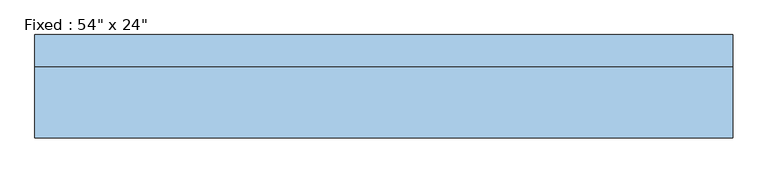
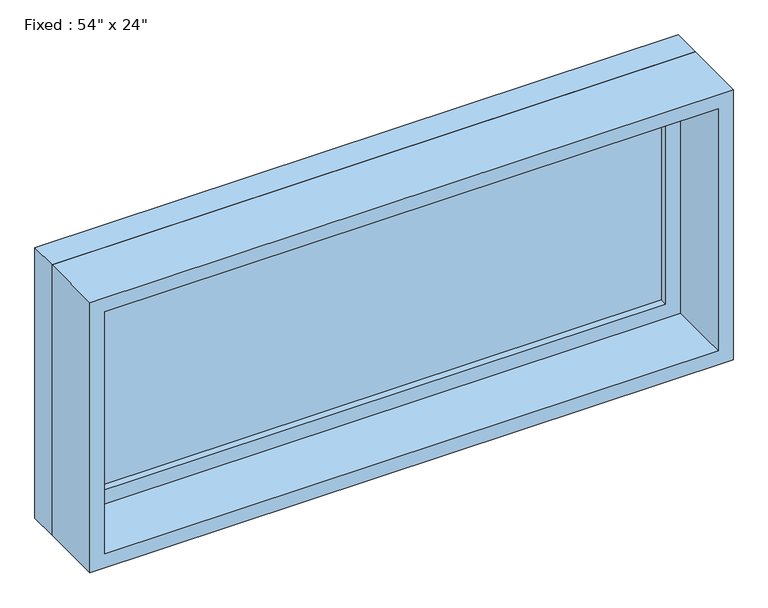
"""IFC4 building model written with IfcOpenShell, lengths in millimetres: window geometry."""

from ifc_helpers import new_model, si_unit, frame, origin, place, context, project, spatial, polyline, outline, extrude, source, transform, mapped, element, save


def window_5b0cf282(model_context):
    return source(origin(), model_context, "Body", "SweptSolid", [
        extrude(outline(polyline([(584.2, 53.975), (-660.4, 53.975), (-660.4, 66.675), (584.2, 66.675), (584.2, 53.975)])), frame((0.0, 0.0, 2197.1), z_axis=(0.0, 0.0, 1.0), x_axis=(1.0, 0.0, 0.0)), (0.0, 0.0, 1.0), 482.6),
        extrude(outline(polyline([(2724.15, -704.85), (2152.65, -704.85), (2152.65, 628.65), (2724.15, 628.65), (2724.15, -704.85)]), holes=[polyline([(2679.7, -660.4), (2679.7, 584.2), (2197.1, 584.2), (2197.1, -660.4), (2679.7, -660.4)])]), frame((0.0, 38.1, 0.0), z_axis=(0.0, 1.0, 0.0), x_axis=(0.0, 0.0, 1.0)), (0.0, 0.0, 1.0), 44.45),
        extrude(outline(polyline([(2743.2, -723.9), (2133.6, -723.9), (2133.6, 647.7), (2743.2, 647.7), (2743.2, -723.9)]), holes=[polyline([(2711.45, -692.15), (2711.45, 615.95), (2165.35, 615.95), (2165.35, -692.15), (2711.45, -692.15)])]), frame((0.0, -101.6, 0.0), z_axis=(0.0, 1.0, 0.0), x_axis=(0.0, 0.0, 1.0)), (0.0, 0.0, 1.0), 139.7),
        extrude(outline(polyline([(2743.2, 647.7), (2743.2, -723.9), (2133.6, -723.9), (2133.6, 647.7), (2743.2, 647.7)]), holes=[polyline([(2724.15, 628.65), (2152.65, 628.65), (2152.65, -704.85), (2724.15, -704.85), (2724.15, 628.65)])]), frame((0.0, 38.1, 0.0), z_axis=(0.0, 1.0, 0.0), x_axis=(0.0, 0.0, 1.0)), (0.0, 0.0, 1.0), 63.5),
    ])


if __name__ == "__main__":
    model = new_model("IFC4")
    model_context = context("Model", 3, world=origin())
    ifc_project = project(units=[si_unit("LENGTHUNIT", "METRE", prefix="MILLI")], contexts=[model_context])
    site = spatial("IfcSite", under=ifc_project)
    building = spatial("IfcBuilding", under=site)
    placement = place(None, origin())
    window_shape = window_5b0cf282(model_context)
    element("IfcWindow", 1, ObjectType="Fixed : 54\" x 24\"", at=placement, inside=building, context=model_context, shape_type="MappedRepresentation", body=[
        mapped(window_shape, transform((0.0, 0.0, 0.0), x_axis=(1.0, 0.0, 0.0), y_axis=(0.0, 1.0, 0.0), z_axis=(0.0, 0.0, 1.0))),
    ])
    save(model, "model.ifc")

# Revit data of these elements
# Type "Fixed : 54\" x 24\""
#   Type Mark = "20"
#   Construction Type Id = "GSP4R"
#   Assembly Code = "B2020100"
#   Analytic Construction = "1/8 in Pilkington single glazing"
#   Visual Light Transmittance = 0.9
#   Solar Heat Gain Coefficient = 0.78
#   Heat Transfer Coefficient (U) = 0.6496 BTU/(h·ft²·°F)
#   Height = 2' - 0"
#   Default Sill Height = 7' - 0"
#   Width = 4' - 6"
#   Window Inset = 0' - 0 3/4"
#   Define Thermal Properties by = 1
#   Glass Pane Material = Glass
#   Sash Material = Sash
#   Wall Closure = (empty or 0)
# Element 1 (IfcWindow, "Fixed : 54\" x 24\"")
#   Materials on its faces: "Sash", "Glass"
# Materials
#   "Glass": class "Glass", colour RGB 0 128 192, transparency 0.75, Description = "Soda Lime Glass", Cost = 0
#   "Sash": class "Wood", colour RGB 224 178 126, transparency 0, Cost = 0
